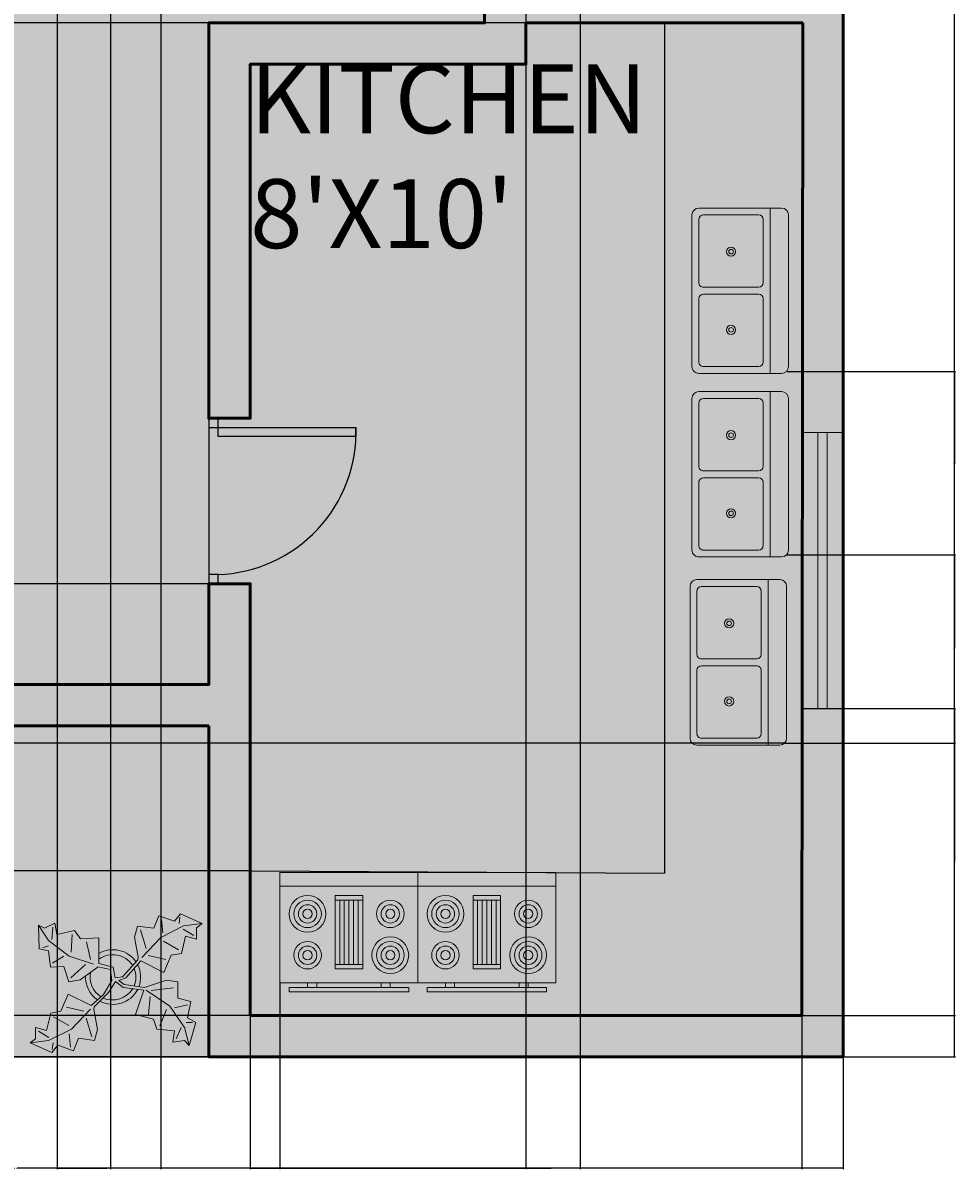
# Model space of a CAD drawing. Units: inches. Extents: x -494 to 1275, y 12 to 1194.
# Tile 2 of 8: x 293 to 496, y 346 to 596. Entities that reach past the tile are written whole.
import ezdxf

# ---------------------------------------------------------------- set-up
doc = ezdxf.new("R2010")
doc.units = ezdxf.units.IN
doc.header["$MEASUREMENT"] = 0
for name, color, linetype, lineweight in [('A-ANNO-DIMS', 2, 'Continuous', 18), ('A-AREA-IDEN', 7, 'Continuous', 25), ('A-DOOR', 3, 'Continuous', 25), ('A-DOOR-PATT', 7, 'Continuous', 13), ('A-EQPM', 8, 'Continuous', 18), ('A-FLOR', 7, 'Continuous', 30), ('A-FLOR-CASE', 7, 'Continuous', 25), ('A-FLOR-FIXT', 8, 'Continuous', 18), ('A-GLAZ', 4, 'Continuous', 18), ('A-GLAZ-FRAM-PATT', 7, 'Continuous', 13), ('A-GLAZ-GLAS-PATT', 4, 'Continuous', 13), ('A-WALL', 7, 'Continuous', 50), ('L-PLNT', 3, 'Continuous', 18)]:
    doc.layers.add(name, color=color, linetype=linetype, lineweight=lineweight)
for name, color, linetype, lineweight, true_color in [('A-FLOR-CASE-PATT', 31, 'Continuous', 13, 0xfecc66), ('A-FLOR-PATT', 51, 'Continuous', 13, 0xf8f6b0), ('A-WALL-PATT', 251, 'Continuous', 13, 0x636466)]:
    doc.layers.add(name, color=color, linetype=linetype, lineweight=lineweight, true_color=true_color)
doc.styles.get("Standard").update_dxf_attribs({"font": 'arial.ttf'})
doc.dimstyles.get("Standard").update_dxf_attribs({"dimtxt": 0.18, "dimasz": 0.18, "dimexe": 0.18, "dimexo": 0.0625, "dimgap": 0.09, "dimtad": 0, "dimtih": 1, "dimtoh": 1, "dimdec": 4, "dimzin": 0, "dimdsep": 46, "dimlunit": 4, "dimtxsty": 'Standard', "dimcen": 0.09, "dimadec": 0, "dimazin": 0, "dimtfac": 1, "dimtdec": 4, "dimtofl": 0, "dimtmove": 0, "dimatfit": 3, "dimfxl": 1, "dimtolj": 1, "dimtzin": 0, "dimarcsym": 0})

# ---------------------------------------------------------------- blocks, each defined once
blk = doc.blocks.new('Range-Oven - 30 in top')
for p, q in [((0, -3), (30, -3)), ((12, -6), (18, -6)), ((13, -20), (13, -6)), ((14, -6), (14, -20)), ((15, -20), (15, -6)), ((16, -6), (16, -20)), ((17, -20), (17, -6)), ((18, -20), (12, -20)), ((6, -24), (6, -25)), ((8, -25), (8, -24)), ((22, -25), (22, -24)), ((24, -24), (24, -25))]:
    blk.add_line(p, q)
for points in [[(0, -24), (0, 0), (30, 0), (30, -24)], [(12, -21), (12, -5), (18, -5), (18, -21)], [(2, -26), (2, -25), (28, -25), (28, -26)]]:
    blk.add_lwpolyline(points, close=True)
for centre, radius in [((6, -9), 4), ((6, -9), 3), ((6, -9), 2), ((24, -9), 3), ((24, -9), 2), ((6, -9), 1), ((24, -9), 1), ((24, -18), 4), ((6, -18), 3), ((6, -18), 2), ((6, -18), 1), ((24, -18), 3), ((24, -18), 2), ((24, -18), 1)]:
    blk.add_circle(centre, radius)
blk = doc.blocks.new('Sink-double - 36 in top')
for p, q in [((-18, -4), (18, -4)), ((-0.75, -18.5), (-0.75, -6.5)), ((0.75, -6.5), (0.75, -18.5))]:
    blk.add_line(p, q)
for points in [[(-16.5, 0), (16.5, 0)], [(-18, -19.5), (-18, -1.5)], [(18, -1.5), (18, -19.5)], [(-16.5, -18.5), (-16.5, -6.5)], [(-15.5, -5.5), (-1.75, -5.5)], [(1.75, -5.5), (15.5, -5.5)], [(16.5, -6.5), (16.5, -18.5)], [(-1.75, -19.5), (-15.5, -19.5)], [(15.5, -19.5), (1.75, -19.5)], [(16.5, -21), (-16.5, -21)]]:
    blk.add_lwpolyline(points)
for centre, radius in [((-8.5, -12.5), 1), ((-8.5, -12.5), 0.5), ((8.5, -12.5), 1), ((8.5, -12.5), 0.5)]:
    blk.add_circle(centre, radius)
for centre, radius, start, end in [((-16.5, -1.5), 1.5, 90, 180), ((16.5, -1.5), 1.5, 0, 90), ((-15.5, -6.5), 1, 90, 180), ((-1.75, -6.5), 1, 0, 90), ((1.75, -6.5), 1, 90, 180), ((15.5, -6.5), 1, 0, 90), ((-16.5, -19.5), 1.5, 180, 270), ((-15.5, -18.5), 1, 180, 270), ((-1.75, -18.5), 1, 270, 0), ((1.75, -18.5), 1, 180, 270), ((15.5, -18.5), 1, 270, 0), ((16.5, -19.5), 1.5, 270, 0)]:
    blk.add_arc(centre, radius, start, end)
blk = doc.blocks.new('WINDOW-60IN')
for p, q in [((3.5, 60), (3.5, 0)), ((5.5, 60), (5.5, 0))]:
    blk.add_line(p, q)
blk.add_lwpolyline([(9, 0), (0, 0), (0, 60), (9, 60)], close=True)
blk = doc.blocks.new('DOOR-SINGLE-36IN')
blk.add_lwpolyline([(34, 2, 0.414214), (2, 32), (4, 32), (4, 2), (2, 2), (2, 32)], format="xyb")
for points in [[(0, 0), (2, 0), (2, 2), (0, 2)], [(34, 0), (36, 0), (36, 2), (34, 2)]]:
    blk.add_lwpolyline(points, close=True)
blk = doc.blocks.new('PLANT-VERANDA')
h = blk.add_hatch(color=256)
h.dxf.hatch_style = 1
h.paths.add_polyline_path([(14.98, 24.96), (10.95, 24.77), (9.63, 26.57), (5.82, 25.7), (5.39, 28.16), (3.14, 27.06), (1.81, 27.74), (1.99, 22.6), (4, 22.14), (4.42, 18.56), (7.33, 18.76), (8.42, 15.4), (10.89, 15.82), (14.48, 18.48), (14.71, 18.7), (17.48, 18.06), (17.78, 15.71), (15.99, 12.65), (13.28, 10.22), (8.28, 12.71), (6.68, 9), (4.49, 8.6), (3.59, 4.8), (1.19, 5.49), (1.2, 2.99), (0, 2.09), (4.7, 0), (6, 1.6), (9.4, 0.41), (10.5, 3.11), (14, 2.62), (14.69, 5.02), (13.88, 9.42), (13.95, 9.99), (17.07, 13.11), (18.6, 15.45), (20.25, 14.18), (24.72, 13.6), (22.95, 8.3), (26.84, 7.24), (27.55, 5.12), (31.44, 4.77), (31.08, 2.29), (33.56, 2.64), (34.62, 1.58), (36.03, 6.53), (34.26, 7.59), (34.97, 11.13), (32.14, 11.84), (32.14, 15.37), (29.67, 15.73), (24.9, 14.15), (20.43, 14.8), (19.31, 15.71), (20.83, 16.24), (24.11, 19.95), (29.12, 17.46), (30.71, 21.17), (32.91, 21.57), (33.8, 25.37), (36.2, 24.68), (36.19, 27.18), (37.39, 28.08), (32.69, 30.17), (31.39, 28.57), (27.99, 29.76), (26.9, 27.06), (23.39, 27.55), (22.7, 25.15), (23.51, 20.75), (23.44, 20.18), (20.12, 16.5), (18.49, 16.24), (18.09, 18.58), (14.94, 19.37)])
h.paths.add_polyline_path([(14.94, 20.36), (14.94, 19.37), (18.09, 18.58), (18.49, 16.24), (20.12, 16.5), (22.33, 18.95, 0.422141)], flags=17)
h.paths.add_polyline_path([(17.78, 15.71), (17.48, 18.06), (14.71, 18.7), (14.48, 18.48), (13.15, 17.5, 0.320154), (15.44, 12.16), (15.99, 12.65)], flags=17)
h.paths.add_polyline_path([(22.35, 13.91), (20.25, 14.18), (18.6, 15.45), (17.07, 13.11), (15.85, 11.88, 0.365185)], flags=17)
h = blk.add_hatch(color=256)
h.dxf.hatch_style = 1
h.paths.add_polyline_path([(13.15, 17.5), (12.06, 16.69, 0.262498), (14.67, 11.47), (15.44, 12.16, -0.320272)])
h.paths.add_polyline_path([(14.95, 21.58), (14.94, 19.37), (18.09, 18.58), (18.49, 16.24), (20.12, 16.5), (23.05, 19.75, 0.39032)])
h = blk.add_hatch(color=256)
h.dxf.hatch_style = 1
h.paths.add_polyline_path([(22.65, 18.29), (20.83, 16.24), (19.31, 15.71), (20.43, 14.8), (22.64, 14.48, 0.196749)])
h.paths.add_polyline_path([(23.39, 19.14), (22.65, 18.29, -0.196749), (22.64, 14.48), (23.64, 14.33, 0.213013)])
h.paths.add_polyline_path([(23.41, 13.77), (20.25, 14.18), (18.6, 15.45), (17.07, 13.11), (15.15, 11.19, 0.412433)])
for p, q in [((31.39, 28.57), (32.69, 30.17)), ((32.69, 30.17), (37.39, 28.08)), ((1.81, 27.74), (4.02, 24.37)), ((1.81, 27.74), (3.14, 27.06)), ((1.99, 22.6), (1.81, 27.74)), ((3.14, 27.06), (5.39, 28.16)), ((5.39, 28.16), (5.82, 25.7)), ((22.7, 25.15), (23.39, 27.55)), ((23.39, 27.55), (26.9, 27.06)), ((26.9, 27.06), (27.99, 29.76)), ((27.99, 29.76), (31.39, 28.57)), ((33.39, 27.57), (28.4, 25.06)), ((28.59, 28.96), (28.9, 26.06)), ((32.59, 29.47), (32.39, 28.07)), ((37.39, 28.08), (33.39, 27.57)), ((37.39, 28.08), (36.19, 27.18)), ((4.69, 24.59), (4.93, 27.27)), ((5.82, 25.7), (9.63, 26.57)), ((9.17, 25.68), (8.92, 21.88)), ((9.63, 26.57), (10.95, 24.77)), ((10.95, 24.77), (14.98, 24.96)), ((14.98, 24.96), (14.94, 19.37)), ((22.7, 25.15), (23.51, 20.75)), ((24, 26.75), (25.21, 22.65)), ((28.4, 25.06), (24.29, 20.67)), ((33.8, 25.37), (32.91, 21.57)), ((33.3, 26.87), (35.6, 25.48)), ((36.2, 24.68), (33.8, 25.37)), ((36.19, 27.18), (36.2, 24.68)), ((4, 22.14), (1.99, 22.6)), ((2.66, 22.82), (4.01, 23.26)), ((4.02, 24.37), (8.46, 20.99)), ((13.16, 20.28), (12.29, 24.09)), ((32.31, 22.37), (29, 24.26)), ((4.42, 18.56), (4, 22.14)), ((4.88, 19.45), (7.35, 20.99)), ((8.46, 20.99), (13.82, 19.26)), ((20.12, 16.5), (23.44, 20.18)), ((23.44, 20.18), (23.51, 20.75)), ((25.71, 21.16), (29.51, 20.26)), ((30.71, 21.17), (29.12, 17.46)), ((32.91, 21.57), (30.71, 21.17)), ((7.33, 18.76), (4.42, 18.56)), ((8.42, 15.4), (7.33, 18.76)), ((8.88, 16.29), (12.03, 19.17)), ((10.89, 15.82), (14.48, 18.48)), ((14.48, 18.48), (14.71, 18.7)), ((14.71, 18.7), (17.48, 18.06)), ((14.94, 19.37), (18.09, 18.58)), ((17.48, 18.06), (17.78, 15.71)), ((17.48, 18.06), (17.48, 18.06)), ((18.09, 18.58), (18.49, 16.24)), ((24.11, 19.95), (20.83, 16.24)), ((29.12, 17.46), (24.11, 19.95)), ((10.89, 15.82), (8.42, 15.4)), ((15.99, 12.65), (17.78, 15.71)), ((17.07, 13.11), (18.6, 15.45)), ((18.49, 16.24), (20.12, 16.5)), ((18.6, 15.45), (20.25, 14.18)), ((20.83, 16.24), (19.31, 15.71)), ((19.31, 15.71), (20.43, 14.8)), ((29.67, 15.73), (24.9, 14.15)), ((29.67, 15.73), (32.14, 15.37)), ((32.14, 15.37), (32.14, 11.84)), ((6.68, 9), (8.28, 12.71)), ((8.28, 12.71), (13.28, 10.22)), ((15.99, 12.65), (13.28, 10.22)), ((13.95, 9.99), (17.07, 13.11)), ((20.25, 14.18), (24.72, 13.6)), ((20.43, 14.8), (24.9, 14.15)), ((22.95, 8.3), (24.72, 13.6)), ((30.38, 10.07), (25.23, 13.59)), ((26.36, 13.52), (31.21, 14.1)), ((13.88, 9.42), (13.95, 9.99)), ((26.13, 12.19), (25.78, 8.3)), ((33.56, 5.47), (30.38, 10.07)), ((34.26, 10.42), (31.44, 9.72)), ((32.14, 11.84), (34.97, 11.13)), ((34.97, 11.13), (34.26, 7.59)), ((3.59, 4.8), (4.49, 8.6)), ((4.49, 8.6), (6.68, 9)), ((5.09, 7.8), (8.39, 5.91)), ((11.68, 9.02), (7.88, 9.91)), ((8.99, 5.11), (13.1, 9.45)), ((13.4, 3.42), (12.19, 7.52)), ((14.69, 5.02), (13.88, 9.42)), ((26.84, 7.24), (22.95, 8.3)), ((28.25, 5.83), (29.67, 9.36)), ((34.26, 7.59), (36.03, 6.53)), ((1.19, 5.49), (3.59, 4.8)), ((1.2, 2.99), (1.19, 5.49)), ((4, 2.6), (8.99, 5.11)), ((14.69, 5.02), (14, 2.62)), ((27.55, 5.12), (26.84, 7.24)), ((31.44, 4.77), (27.55, 5.12)), ((32.85, 5.47), (31.79, 3)), ((34.62, 1.58), (33.56, 5.47)), ((35.33, 6.53), (33.91, 6.53)), ((36.03, 6.53), (34.62, 1.58)), ((0, 2.09), (1.2, 2.99)), ((0, 2.09), (4, 2.6)), ((4.1, 3.3), (1.79, 4.69)), ((8.8, 1.21), (8.5, 4.11)), ((10.5, 3.11), (9.4, 0.41)), ((14, 2.62), (10.5, 3.11)), ((31.08, 2.29), (31.44, 4.77)), ((33.56, 2.64), (31.08, 2.29)), ((34.62, 1.58), (33.56, 2.64)), ((4.7, 0), (0, 2.09)), ((6, 1.6), (4.7, 0)), ((4.8, 0.7), (5, 2.1)), ((9.4, 0.41), (6, 1.6))]:
    blk.add_line(p, q)
for centre, radius, start, end in [((18.01, 16.27), 6.13, 34.3757, 120.1028), ((17.95, 16.06), 5.25, 33.8219, 124.9414), ((18.04, 16.43), 5, 167.6804, 238.6774), ((17.99, 16.39), 5.03, 337.6469, 22.1698), ((18.14, 16.45), 5.9, 338.9388, 27.0389), ((18, 16.4), 5.94, 177.1741, 236.0068), ((17.98, 16.63), 6.14, 242.5292, 332.1842), ((17.9, 16.76), 5.29, 247.3711, 327.472)]:
    blk.add_arc(centre, radius, start, end)
blk = doc.blocks.new('*D42')
at = {"layer": 'A-ANNO-DIMS', "color": 0, "lineweight": -2, "transparency": 16777216}
for p, q in [((111.73, 370.47), (111.73, 346.1)), ((471.73, 370.47), (471.73, 346.1)), ((111.91, 346.28), (291.44, 346.28)), ((471.55, 346.28), (292.02, 346.28))]:
    blk.add_line(p, q, dxfattribs=at)
at = {"layer": 'A-ANNO-DIMS', "color": 0, "transparency": 16777216}
for points in [[(111.91, 346.31), (111.91, 346.25), (111.73, 346.28)], [(471.55, 346.31), (471.55, 346.25), (471.73, 346.28)]]:
    blk.add_solid(points, dxfattribs=at)
at = {"layer": 'Defpoints', "color": 0, "transparency": 16777216}
for p in [(111.73, 370.53), (471.73, 370.53), (471.73, 346.28)]:
    blk.add_point(p, dxfattribs=at)
at = {"layer": 'A-ANNO-DIMS', "color": 0, "transparency": 16777216, "insert": (291.73, 346.28), "char_height": 0.18, "attachment_point": 5}
blk.add_mtext('\\A1;360', dxfattribs=at)
blk = doc.blocks.new('*D43')
at = {"layer": 'A-ANNO-DIMS', "color": 0, "lineweight": -2, "transparency": 16777216}
for p, q in [((471.79, 850.53), (496.16, 850.53)), ((495.98, 850.35), (495.98, 610.72)), ((495.98, 370.71), (495.98, 610.35)), ((471.79, 370.53), (496.16, 370.53))]:
    blk.add_line(p, q, dxfattribs=at)
at = {"layer": 'A-ANNO-DIMS', "color": 0, "transparency": 16777216}
for points in [[(495.95, 850.35), (496.01, 850.35), (495.98, 850.53)], [(495.95, 370.71), (496.01, 370.71), (495.98, 370.53)]]:
    blk.add_solid(points, dxfattribs=at)
at = {"layer": 'Defpoints', "color": 0, "transparency": 16777216}
for p in [(471.73, 850.53), (495.98, 850.53), (471.73, 370.53)]:
    blk.add_point(p, dxfattribs=at)
at = {"layer": 'A-ANNO-DIMS', "color": 0, "transparency": 16777216, "insert": (495.98, 610.53), "char_height": 0.18, "attachment_point": 5}
blk.add_mtext('\\A1;480', dxfattribs=at)
blk = doc.blocks.new('*D53')
at = {"layer": 'A-ANNO-DIMS', "color": 0, "lineweight": -2, "transparency": 16777216}
for p, q in [((300.73, 697.47), (300.73, 346.1)), ((312.31, 688.47), (312.31, 346.1)), ((300.91, 346.28), (306.07, 346.28)), ((312.13, 346.28), (306.98, 346.28))]:
    blk.add_line(p, q, dxfattribs=at)
at = {"layer": 'A-ANNO-DIMS', "color": 0, "transparency": 16777216}
for points in [[(300.91, 346.31), (300.91, 346.25), (300.73, 346.28)], [(312.13, 346.31), (312.13, 346.25), (312.31, 346.28)]]:
    blk.add_solid(points, dxfattribs=at)
at = {"layer": 'Defpoints', "color": 0, "transparency": 16777216}
for p in [(300.73, 697.53), (312.31, 688.53), (312.31, 346.28)]:
    blk.add_point(p, dxfattribs=at)
at = {"layer": 'A-ANNO-DIMS', "color": 0, "transparency": 16777216, "insert": (306.52, 346.28), "char_height": 0.18, "attachment_point": 5}
blk.add_mtext('\\A1;11.577', dxfattribs=at)
blk = doc.blocks.new('*D57')
at = {"layer": 'A-ANNO-DIMS', "color": 0, "lineweight": -2, "transparency": 16777216}
for p, q in [((462.79, 446.37), (496.16, 446.37)), ((495.98, 446.19), (495.98, 413.14)), ((495.98, 379.71), (495.98, 412.77)), ((462.8, 379.53), (496.16, 379.53))]:
    blk.add_line(p, q, dxfattribs=at)
at = {"layer": 'A-ANNO-DIMS', "color": 0, "transparency": 16777216}
for points in [[(495.95, 446.19), (496.01, 446.19), (495.98, 446.37)], [(495.95, 379.71), (496.01, 379.71), (495.98, 379.53)]]:
    blk.add_solid(points, dxfattribs=at)
at = {"layer": 'Defpoints', "color": 0, "transparency": 16777216}
for p in [(462.73, 446.37), (495.98, 446.37), (462.74, 379.53)]:
    blk.add_point(p, dxfattribs=at)
at = {"layer": 'A-ANNO-DIMS', "color": 0, "transparency": 16777216, "insert": (495.98, 412.95), "char_height": 0.18, "attachment_point": 5}
blk.add_mtext('\\A1;66.84', dxfattribs=at)
blk = doc.blocks.new('*D59')
at = {"layer": 'A-ANNO-DIMS', "color": 0, "lineweight": -2, "transparency": 16777216}
for p, q in [((342.67, 473.5), (87.3, 473.5)), ((87.48, 473.32), (87.48, 426.7)), ((87.48, 379.71), (87.48, 426.33)), ((342.67, 379.53), (87.3, 379.53))]:
    blk.add_line(p, q, dxfattribs=at)
at = {"layer": 'A-ANNO-DIMS', "color": 0, "transparency": 16777216}
for points in [[(87.45, 473.32), (87.51, 473.32), (87.48, 473.5)], [(87.45, 379.71), (87.51, 379.71), (87.48, 379.53)]]:
    blk.add_solid(points, dxfattribs=at)
at = {"layer": 'Defpoints', "color": 0, "transparency": 16777216}
for p in [(87.48, 473.5), (342.73, 473.5), (342.73, 379.53)]:
    blk.add_point(p, dxfattribs=at)
at = {"layer": 'A-ANNO-DIMS', "color": 0, "transparency": 16777216, "insert": (87.48, 426.52), "char_height": 0.18, "attachment_point": 5}
blk.add_mtext('\\A1;93.96', dxfattribs=at)
blk = doc.blocks.new('*D60')
at = {"layer": 'A-ANNO-DIMS', "color": 0, "lineweight": -2, "transparency": 16777216}
for p, q in [((342.73, 379.47), (342.73, 346.1)), ((462.74, 379.47), (462.74, 346.1)), ((342.91, 346.28), (402.46, 346.28)), ((462.56, 346.28), (403.02, 346.28))]:
    blk.add_line(p, q, dxfattribs=at)
at = {"layer": 'A-ANNO-DIMS', "color": 0, "transparency": 16777216}
for points in [[(342.91, 346.31), (342.91, 346.25), (342.73, 346.28)], [(462.56, 346.31), (462.56, 346.25), (462.74, 346.28)]]:
    blk.add_solid(points, dxfattribs=at)
at = {"layer": 'Defpoints', "color": 0, "transparency": 16777216}
for p in [(342.73, 379.53), (462.74, 379.53), (342.73, 346.28)]:
    blk.add_point(p, dxfattribs=at)
at = {"layer": 'A-ANNO-DIMS', "color": 0, "transparency": 16777216, "insert": (402.74, 346.28), "char_height": 0.18, "attachment_point": 5}
blk.add_mtext('\\A1;120', dxfattribs=at)
blk = doc.blocks.new('*D63')
at = {"layer": 'A-ANNO-DIMS', "color": 0, "lineweight": -2, "transparency": 16777216}
for p, q in [((402.67, 595.53), (87.3, 595.53)), ((87.48, 595.35), (87.48, 487.72)), ((87.48, 379.71), (87.48, 487.35)), ((342.67, 379.53), (87.3, 379.53))]:
    blk.add_line(p, q, dxfattribs=at)
at = {"layer": 'A-ANNO-DIMS', "color": 0, "transparency": 16777216}
for points in [[(87.45, 595.35), (87.51, 595.35), (87.48, 595.53)], [(87.45, 379.71), (87.51, 379.71), (87.48, 379.53)]]:
    blk.add_solid(points, dxfattribs=at)
at = {"layer": 'Defpoints', "color": 0, "transparency": 16777216}
for p in [(402.73, 595.53), (87.48, 379.53), (342.73, 379.53)]:
    blk.add_point(p, dxfattribs=at)
at = {"layer": 'A-ANNO-DIMS', "color": 0, "transparency": 16777216, "insert": (87.48, 487.53), "char_height": 0.18, "attachment_point": 5}
blk.add_mtext('\\A1;216', dxfattribs=at)
blk = doc.blocks.new('*D65')
at = {"layer": 'A-ANNO-DIMS', "color": 0, "lineweight": -2, "transparency": 16777216}
for p, q in [((459.46, 479.75), (496.16, 479.75)), ((495.98, 479.57), (495.98, 459.47)), ((495.98, 439), (495.98, 459.1)), ((459.04, 438.82), (496.16, 438.82))]:
    blk.add_line(p, q, dxfattribs=at)
at = {"layer": 'A-ANNO-DIMS', "color": 0, "transparency": 16777216}
for points in [[(495.95, 479.57), (496.01, 479.57), (495.98, 479.75)], [(495.95, 439), (496.01, 439), (495.98, 438.82)]]:
    blk.add_solid(points, dxfattribs=at)
at = {"layer": 'Defpoints', "color": 0, "transparency": 16777216}
for p in [(459.4, 479.75), (495.98, 479.75), (458.98, 438.82)]:
    blk.add_point(p, dxfattribs=at)
at = {"layer": 'A-ANNO-DIMS', "color": 0, "transparency": 16777216, "insert": (495.98, 459.28), "char_height": 0.18, "attachment_point": 5}
blk.add_mtext('\\A1;40.93', dxfattribs=at)
blk = doc.blocks.new('*D66')
at = {"layer": 'A-ANNO-DIMS', "color": 0, "lineweight": -2, "transparency": 16777216}
for p, q in [((459.46, 519.69), (496.16, 519.69)), ((495.98, 519.51), (495.98, 499.9)), ((495.98, 479.93), (495.98, 499.54)), ((459.46, 479.75), (496.16, 479.75))]:
    blk.add_line(p, q, dxfattribs=at)
at = {"layer": 'A-ANNO-DIMS', "color": 0, "transparency": 16777216}
for points in [[(495.95, 519.51), (496.01, 519.51), (495.98, 519.69)], [(495.95, 479.93), (496.01, 479.93), (495.98, 479.75)]]:
    blk.add_solid(points, dxfattribs=at)
at = {"layer": 'Defpoints', "color": 0, "transparency": 16777216}
for p in [(459.4, 519.69), (495.98, 519.69), (459.4, 479.75)]:
    blk.add_point(p, dxfattribs=at)
at = {"layer": 'A-ANNO-DIMS', "color": 0, "transparency": 16777216, "insert": (495.98, 499.72), "char_height": 0.18, "attachment_point": 5}
blk.add_mtext('\\A1;39.94', dxfattribs=at)
blk = doc.blocks.new('*D67')
at = {"layer": 'A-ANNO-DIMS', "color": 0, "lineweight": -2, "transparency": 16777216}
for p, q in [((349.21, 386.58), (349.21, 346.1)), ((342.73, 379.47), (342.73, 346.1)), ((342.91, 346.28), (345.65, 346.28)), ((349.03, 346.28), (346.3, 346.28))]:
    blk.add_line(p, q, dxfattribs=at)
at = {"layer": 'A-ANNO-DIMS', "color": 0, "transparency": 16777216}
for points in [[(342.91, 346.31), (342.91, 346.25), (342.73, 346.28)], [(349.03, 346.31), (349.03, 346.25), (349.21, 346.28)]]:
    blk.add_solid(points, dxfattribs=at)
at = {"layer": 'Defpoints', "color": 0, "transparency": 16777216}
for p in [(349.21, 386.65), (342.73, 379.53), (349.21, 346.28)]:
    blk.add_point(p, dxfattribs=at)
at = {"layer": 'A-ANNO-DIMS', "color": 0, "transparency": 16777216, "insert": (345.97, 346.28), "char_height": 0.18, "attachment_point": 5}
blk.add_mtext('\\A1;6.48', dxfattribs=at)
blk = doc.blocks.new('*D68')
at = {"layer": 'A-ANNO-DIMS', "color": 0, "lineweight": -2, "transparency": 16777216}
for p, q in [((458.91, 438.82), (87.3, 438.82)), ((87.48, 438.64), (87.48, 409.36)), ((87.48, 379.71), (87.48, 408.99)), ((462.68, 379.53), (87.3, 379.53))]:
    blk.add_line(p, q, dxfattribs=at)
at = {"layer": 'A-ANNO-DIMS', "color": 0, "transparency": 16777216}
for points in [[(87.45, 438.64), (87.51, 438.64), (87.48, 438.82)], [(87.45, 379.71), (87.51, 379.71), (87.48, 379.53)]]:
    blk.add_solid(points, dxfattribs=at)
at = {"layer": 'Defpoints', "color": 0, "transparency": 16777216}
for p in [(87.48, 438.82), (458.98, 438.82), (462.74, 379.53)]:
    blk.add_point(p, dxfattribs=at)
at = {"layer": 'A-ANNO-DIMS', "color": 0, "transparency": 16777216, "insert": (87.48, 409.18), "char_height": 0.18, "attachment_point": 5}
blk.add_mtext('\\A1;59.28', dxfattribs=at)
blk = doc.blocks.new('*D69')
at = {"layer": 'A-ANNO-DIMS', "color": 0, "lineweight": -2, "transparency": 16777216}
for p, q in [((402.73, 604.47), (402.73, 346.1)), ((414.52, 604.78), (414.52, 346.1)), ((402.91, 346.28), (408.19, 346.28)), ((414.34, 346.28), (409.07, 346.28))]:
    blk.add_line(p, q, dxfattribs=at)
at = {"layer": 'A-ANNO-DIMS', "color": 0, "transparency": 16777216}
for points in [[(402.91, 346.31), (402.91, 346.25), (402.73, 346.28)], [(414.34, 346.31), (414.34, 346.25), (414.52, 346.28)]]:
    blk.add_solid(points, dxfattribs=at)
at = {"layer": 'Defpoints', "color": 0, "transparency": 16777216}
for p in [(402.73, 604.53), (414.52, 604.84), (414.52, 346.28)]:
    blk.add_point(p, dxfattribs=at)
at = {"layer": 'A-ANNO-DIMS', "color": 0, "transparency": 16777216, "insert": (408.63, 346.28), "char_height": 0.18, "attachment_point": 5}
blk.add_mtext('\\A1;11.791', dxfattribs=at)
blk = doc.blocks.new('*D83')
at = {"layer": 'A-ANNO-DIMS', "color": 0, "lineweight": -2, "transparency": 16777216}
for p, q in [((300.73, 820.48), (300.73, 346.1)), ((323.29, 820.48), (323.29, 346.1)), ((300.91, 346.28), (311.55, 346.28)), ((323.11, 346.28), (312.48, 346.28))]:
    blk.add_line(p, q, dxfattribs=at)
at = {"layer": 'A-ANNO-DIMS', "color": 0, "transparency": 16777216}
for points in [[(300.91, 346.31), (300.91, 346.25), (300.73, 346.28)], [(323.11, 346.31), (323.11, 346.25), (323.29, 346.28)]]:
    blk.add_solid(points, dxfattribs=at)
at = {"layer": 'Defpoints', "color": 0, "transparency": 16777216}
for p in [(300.73, 820.54), (323.29, 820.54), (323.29, 346.28)]:
    blk.add_point(p, dxfattribs=at)
at = {"layer": 'A-ANNO-DIMS', "color": 0, "transparency": 16777216, "insert": (312.01, 346.28), "char_height": 0.18, "attachment_point": 5}
blk.add_mtext('\\A1;22.557', dxfattribs=at)
blk = doc.blocks.new('*D97')
at = {"layer": 'A-ANNO-DIMS', "color": 0, "lineweight": -2, "transparency": 16777216}
for p, q in [((342.67, 411.03), (87.3, 411.03)), ((87.48, 410.85), (87.48, 395.47)), ((87.48, 379.71), (87.48, 395.1)), ((342.67, 379.53), (87.3, 379.53))]:
    blk.add_line(p, q, dxfattribs=at)
at = {"layer": 'A-ANNO-DIMS', "color": 0, "transparency": 16777216}
for points in [[(87.45, 410.85), (87.51, 410.85), (87.48, 411.03)], [(87.45, 379.71), (87.51, 379.71), (87.48, 379.53)]]:
    blk.add_solid(points, dxfattribs=at)
at = {"layer": 'Defpoints', "color": 0, "transparency": 16777216}
for p in [(342.73, 411.03), (87.48, 379.53), (342.73, 379.53)]:
    blk.add_point(p, dxfattribs=at)
at = {"layer": 'A-ANNO-DIMS', "color": 0, "transparency": 16777216, "insert": (87.48, 395.28), "char_height": 0.18, "attachment_point": 5}
blk.add_mtext('\\A1;31.5', dxfattribs=at)

msp = doc.modelspace()

# ---------------------------------------------------------------- hatches: boundary and pattern name
at = {"layer": 'A-DOOR-PATT'}
h = msp.add_hatch(color=256, dxfattribs=at)
h.dxf.hatch_style = 1
h.paths.add_polyline_path([(365.7322, 505.4986), (365.7322, 507.4986), (335.7322, 507.4986), (335.7322, 505.4986)])
h.paths.add_polyline_path([(335.7322, 507.4986), (335.7322, 509.4986), (333.7322, 509.4986), (333.7322, 507.4986)])
h.paths.add_polyline_path([(335.7322, 473.4986), (335.7322, 475.4986), (333.7322, 475.4986), (333.7322, 473.4986)])
at = {"layer": 'A-FLOR-CASE-PATT'}
h = msp.add_hatch(color=256, dxfattribs=at)
h.dxf.hatch_style = 1
h.paths.add_polyline_path([(462.8026, 446.3728), (462.7322, 446.3728), (462.7322, 506.3728), (462.9409, 595.5349), (432.8366, 595.5349), (432.8366, 410.5086), (342.7322, 411.0349), (342.7322, 379.5349), (462.7406, 379.5349)])
at = {"layer": 'A-FLOR-PATT'}
h = msp.add_hatch(color=256, dxfattribs=at)
h.dxf.hatch_style = 1
h.paths.add_polyline_path([(333.7322, 595.5349), (393.7322, 595.5349), (393.7322, 617.1185), (393.7322, 653.1185), (393.7322, 688.5349), (348.3096, 688.5349), (348.3096, 697.5349), (462.7322, 697.5349), (462.7322, 841.5349), (300.7322, 841.5349), (300.7322, 820.5433), (323.2889, 820.5433), (323.2889, 769.5349), (300.7322, 769.5349), (300.7322, 697.5349), (312.3096, 697.5349), (312.3096, 688.5349), (276.4565, 688.5349), (276.4565, 697.5349), (291.7322, 697.5349), (291.7322, 771.5415), (264.338, 771.5415), (264.338, 820.5433), (291.7322, 820.5433), (291.7322, 841.5349), (120.7322, 841.5349), (120.7322, 697.5349), (240.4565, 697.5349), (240.4565, 688.5349), (120.7322, 688.5349), (120.7322, 451.5349), (241.3385, 451.5349), (241.3385, 442.5349), (277.3385, 442.5349), (277.3385, 451.5349), (333.7322, 451.5349), (333.7322, 473.4986), (333.7322, 509.4986)])
h.paths.add_polyline_path([(372.4977, 745.1275), (372.4977, 805.1275), (452.4977, 805.1275), (452.4977, 745.1275)], flags=16)
h.paths.add_polyline_path([(208.4976, 745.1275), (128.4976, 745.1275), (128.4976, 805.1275), (208.4976, 805.1275)], flags=16)
h.paths.add_polyline_path([(422.8977, 745.1275), (422.8977, 760.3275), (438.0977, 760.3275), (438.0977, 797.1275), (451.2977, 797.1275), (451.2977, 776.3275), (438.0977, 776.3275), (438.0977, 773.9275), (451.2977, 773.9275), (451.2977, 753.1275), (436.0977, 753.1275), (436.0977, 758.3275)], flags=16)
h.paths.add_polyline_path([(142.8976, 789.9275), (142.8976, 753.1275), (129.6976, 753.1275), (129.6976, 773.9275), (142.8976, 773.9275), (142.8976, 776.3275), (129.6976, 776.3275), (129.6976, 797.1275), (144.8976, 797.1275), (144.8976, 791.9275), (158.0976, 805.1275), (158.0976, 789.9275)], flags=0)
h = msp.add_hatch(color=256, dxfattribs=at)
h.dxf.hatch_style = 1
h.paths.add_polyline_path([(432.8366, 595.5349), (402.7322, 595.5349), (402.7322, 586.5349), (393.7322, 586.5349), (342.7322, 586.5349), (342.7322, 509.4986), (342.7322, 473.4986), (342.7322, 442.5349), (342.7322, 411.0349), (432.8366, 410.5086)])
h = msp.add_hatch(color=256, dxfattribs=at)
h.dxf.hatch_style = 1
h.paths.add_polyline_path([(342.7322, 509.4986), (333.7322, 509.4986), (333.7322, 473.4986), (342.7322, 473.4986)])
h = msp.add_hatch(color=256, dxfattribs=at)
h.dxf.hatch_style = 1
h.paths.add_polyline_path([(333.7322, 442.5349), (277.3385, 442.5349), (241.3385, 442.5349), (111.7322, 442.5349), (111.7322, 370.5349), (333.7322, 370.5349)])
at = {"layer": 'A-GLAZ-FRAM-PATT'}
h = msp.add_hatch(color=256, dxfattribs=at)
h.dxf.hatch_style = 1
h.paths.add_polyline_path([(468.2322, 446.3728), (471.7322, 446.3728), (471.7322, 506.3728), (468.2322, 506.3728)])
h.paths.add_polyline_path([(466.2322, 506.3728), (462.7322, 506.3728), (462.7322, 446.3728), (466.2322, 446.3728)])
at = {"layer": 'A-GLAZ-GLAS-PATT'}
h = msp.add_hatch(color=256, dxfattribs=at)
h.dxf.hatch_style = 1
h.paths.add_polyline_path([(468.2322, 506.3728), (466.2322, 506.3728), (466.2322, 446.3728), (468.2322, 446.3728)])
at = {"layer": 'A-WALL-PATT'}
h = msp.add_hatch(color=256, dxfattribs=at)
h.dxf.hatch_style = 1
h.paths.add_polyline_path([(120.7322, 841.5349), (291.7322, 841.5349), (291.7322, 697.5349), (276.4565, 697.5349), (276.4565, 688.5349), (312.3096, 688.5349), (312.3096, 697.5349), (300.7322, 697.5349), (300.7322, 841.5349), (462.7322, 841.5349), (462.7322, 697.5349), (348.3096, 697.5349), (348.3096, 688.5349), (393.7322, 688.5349), (393.7322, 653.1185), (402.7322, 653.1185), (402.7322, 688.5349), (462.7322, 688.5349), (462.7322, 604.5349), (402.7322, 604.5349), (402.7322, 617.1185), (393.7322, 617.1185), (393.7322, 595.5349), (333.7322, 595.5349), (333.7322, 509.4986), (342.7322, 509.4986), (342.7322, 586.5349), (393.7322, 586.5349), (402.7322, 586.5349), (402.7322, 595.5349), (462.9409, 595.5349), (462.7406, 379.5349), (342.7322, 379.5349), (342.7322, 442.5349), (342.7322, 473.4986), (333.7322, 473.4986), (333.7322, 451.5349), (277.3385, 451.5349), (277.3385, 442.5349), (333.7322, 442.5349), (333.7322, 370.5349), (471.7322, 370.5349), (471.7322, 850.5349), (111.7322, 850.5349), (111.7322, 442.5349), (241.3385, 442.5349), (241.3385, 451.5349), (120.7322, 451.5349), (120.7322, 688.5349), (240.4565, 688.5349), (240.4565, 697.5349), (120.7322, 697.5349)])

# ---------------------------------------------------------------- linework, layer by layer
at = {"layer": 'A-DOOR'}
msp.add_line((333.7322, 509.4986), (333.7322, 473.4986), dxfattribs=at)
msp.add_line((333.7322, 509.4986), (333.7322, 473.4986), dxfattribs=at)
at = {"layer": 'A-FLOR'}
msp.add_line((111.7322, 370.5349), (333.7322, 370.5349), dxfattribs=at)
at = {"layer": 'A-FLOR-CASE'}
for p in [(432.8366, 595.5349), (342.7322, 411.0349)]:
    msp.add_line(p, (432.8366, 410.5086), dxfattribs=at)
at = {"layer": 'A-WALL'}
for points in [[(333.7322, 442.5349), (333.7322, 370.5349), (471.7322, 370.5349), (471.7322, 850.5349), (111.7322, 850.5349), (111.7322, 442.5349), (241.3385, 442.5349), (241.3385, 451.5349), (120.7322, 451.5349), (120.7322, 688.5349), (240.4565, 688.5349), (240.4565, 697.5349), (120.7322, 697.5349), (120.7322, 841.5349), (291.7322, 841.5349), (291.7322, 697.5349), (276.4565, 697.5349), (276.4565, 688.5349), (312.3096, 688.5349), (312.3096, 697.5349), (300.7322, 697.5349), (300.7322, 841.5349)], [(462.9409, 595.5349), (402.7322, 595.5349), (402.7322, 586.5349), (393.7322, 586.5349), (342.7322, 586.5349), (342.7322, 509.4986), (333.7322, 509.4986), (333.7322, 595.5349), (393.7322, 595.5349), (393.7322, 617.1185), (402.7322, 617.1185), (402.7322, 604.5349), (462.7322, 604.5349), (462.7322, 688.5349), (402.7322, 688.5349), (402.7322, 653.1185), (393.7322, 653.1185), (393.7322, 688.5349), (348.3096, 688.5349), (348.3096, 697.5349), (462.7322, 697.5349), (462.7322, 841.5349), (300.7322, 841.5349)], [(333.7322, 442.5349), (277.3385, 442.5349), (277.3385, 451.5349), (333.7322, 451.5349), (333.7322, 473.4986), (342.7322, 473.4986), (342.7322, 442.5349), (342.7322, 379.5349), (462.7406, 379.5349), (462.9409, 595.5349)]]:
    msp.add_lwpolyline(points, dxfattribs=at)

# ---------------------------------------------------------------- block references
at = {"layer": 'A-DOOR', "rotation": 269.9999999999999}
msp.add_blockref('DOOR-SINGLE-36IN', (333.7323, 509.4983), dxfattribs=at)
at = {"layer": 'A-EQPM'}
for p in [(349.2128, 410.6466), (379.2128, 410.6466)]:
    msp.add_blockref('Range-Oven - 30 in top', p, dxfattribs=at)
at = {"layer": 'A-FLOR-FIXT', "rotation": 270}
for p in [(459.8404, 537.2524), (459.8404, 497.3111), (459.4152, 456.3793)]:
    msp.add_blockref('Sink-double - 36 in top', p, dxfattribs=at)
at = {"layer": 'A-GLAZ'}
msp.add_blockref('WINDOW-60IN', (462.7319, 446.3732), dxfattribs=at)
at = {"layer": 'L-PLNT'}
msp.add_blockref('PLANT-VERANDA', (294.8613, 371.4527), dxfattribs=at)

# ---------------------------------------------------------------- texts
at = {"layer": 'A-AREA-IDEN', "insert": (342.7322, 586.5349), "char_height": 15, "attachment_point": 1}
msp.add_mtext_dynamic_manual_height_columns("KITCHEN\\P8'X10'", width=90.104365, gutter_width=1, heights=[0], dxfattribs=at)

# ---------------------------------------------------------------- dimensions: what is measured, and where the dimension line sits
at = {"layer": 'A-ANNO-DIMS'}
for base, p1, p2, override, picture, middle in [((495.9822, 850.5349), (471.7322, 370.5349), (471.7322, 850.5349), {"dimdec": 0, "dimlfac": 1, "dimrnd": 0, "dimzin": 0, "dimdsep": 46, "dimlunit": 2}, '*D43', (495.9822, 610.5349)), ((87.4822, 379.5349), (402.7322, 595.5349), (342.7322, 379.5349), {"dimdec": 0, "dimlfac": 1, "dimrnd": 0, "dimzin": 0, "dimdsep": 46, "dimlunit": 2}, '*D63', (87.4822, 487.5349)), ((495.9822, 519.6917), (459.4011, 479.7505), (459.4011, 519.6917), {"dimdec": 2, "dimlfac": 1, "dimrnd": 0, "dimzin": 0, "dimdsep": 46, "dimlunit": 2}, '*D66', (495.9822, 499.7211)), ((495.9822, 479.7505), (458.9758, 438.8186), (459.4011, 479.7505), {"dimdec": 2, "dimlfac": 1, "dimrnd": 0, "dimzin": 0, "dimdsep": 46, "dimlunit": 2}, '*D65', (495.9822, 459.2845)), ((87.4822, 473.4986), (342.7322, 379.5349), (342.7322, 473.4986), {"dimdec": 2, "dimlfac": 1, "dimrnd": 0, "dimzin": 0, "dimdsep": 46, "dimlunit": 2}, '*D59', (87.4822, 426.5167)), ((495.9822, 446.3728), (462.7406, 379.5349), (462.7322, 446.3728), {"dimdec": 2, "dimlfac": 1, "dimrnd": 0, "dimzin": 0, "dimdsep": 46, "dimlunit": 2}, '*D57', (495.9822, 412.9538)), ((87.4822, 438.8186), (462.7406, 379.5349), (458.9758, 438.8186), {"dimdec": 2, "dimlfac": 1, "dimrnd": 0, "dimzin": 0, "dimdsep": 46, "dimlunit": 2}, '*D68', (87.4822, 409.1768)), ((87.4822, 379.5349), (342.7322, 411.0349), (342.7322, 379.5349), {"dimdec": 1, "dimlfac": 1, "dimrnd": 0, "dimzin": 0, "dimdsep": 46, "dimlunit": 2}, '*D97', (87.4822, 395.2849))]:
    dim = msp.add_linear_dim(base=base, p1=p1, p2=p2, angle=90, dimstyle='Standard', override=override, dxfattribs=at)
    dim.commit()
    dim.dimension.update_dxf_attribs({"geometry": picture, "text_midpoint": middle})
for base, p1, p2, override, picture, middle in [((323.2889, 346.2849), (300.7322, 820.5433), (323.2889, 820.5433), {"dimdec": 3, "dimlfac": 1, "dimrnd": 0, "dimzin": 0, "dimdsep": 46, "dimlunit": 2}, '*D83', (312.0106, 346.2849)), ((312.3096, 346.2849), (300.7322, 697.5349), (312.3096, 688.5349), {"dimdec": 3, "dimlfac": 1, "dimrnd": 0, "dimzin": 0, "dimdsep": 46, "dimlunit": 2}, '*D53', (306.5209, 346.2849)), ((414.5234, 346.2849), (402.7322, 604.5349), (414.5234, 604.8376), {"dimdec": 3, "dimlfac": 1, "dimrnd": 0, "dimzin": 0, "dimdsep": 46, "dimlunit": 2}, '*D69', (408.6278, 346.2849)), ((349.2128, 346.2849), (342.7322, 379.5349), (349.2128, 386.6466), {"dimdec": 2, "dimlfac": 1, "dimrnd": 0, "dimzin": 0, "dimdsep": 46, "dimlunit": 2}, '*D67', (345.9725, 346.2849)), ((342.7322, 346.2849), (462.7406, 379.5349), (342.7322, 379.5349), {"dimdec": 0, "dimlfac": 1, "dimrnd": 0, "dimzin": 0, "dimdsep": 46, "dimlunit": 2}, '*D60', (402.7364, 346.2849)), ((471.7322, 346.2849), (111.7322, 370.5349), (471.7322, 370.5349), {"dimdec": 0, "dimlfac": 1, "dimrnd": 0, "dimzin": 0, "dimdsep": 46, "dimlunit": 2}, '*D42', (291.7322, 346.2849))]:
    dim = msp.add_linear_dim(base=base, p1=p1, p2=p2, dimstyle='Standard', override=override, dxfattribs=at)
    dim.commit()
    dim.dimension.update_dxf_attribs({"geometry": picture, "text_midpoint": middle})

doc.saveas('drawing.dxf')
